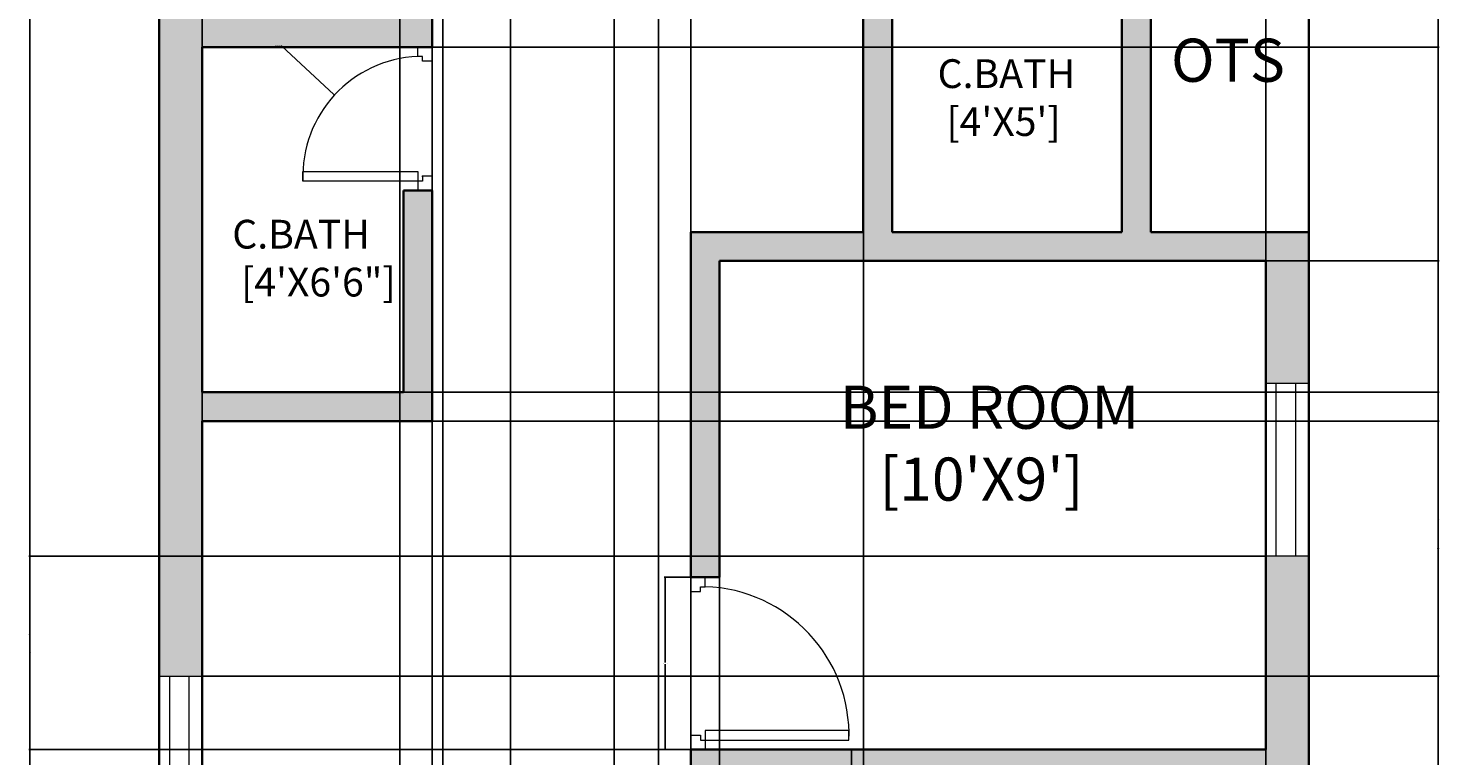
# Model space of a CAD drawing. Units: inches. Extents: x 1963 to 2258, y 1522 to 2116.
# Tile 2 of 3: x 1963 to 2257, y 1793 to 1945. Entities that reach past the tile are written whole.
import ezdxf

# ---------------------------------------------------------------- set-up
doc = ezdxf.new("R2010")
doc.units = ezdxf.units.IN
for name, color, linetype, lineweight in [('A-ANNO-DIMS', 2, 'Continuous', 18), ('A-AREA-IDEN', 7, 'Continuous', 18), ('A-DOOR', 3, 'Continuous', 18), ('A-GLAZ', 4, 'Continuous', 18), ('A-WALL', 7, 'Continuous', 35), ('A-WALL-PATT', 250, 'Continuous', 13)]:
    doc.layers.add(name, color=color, linetype=linetype, lineweight=lineweight)
doc.styles.get("Standard").update_dxf_attribs({"font": 'arial.ttf'})
doc.dimstyles.get("Standard").update_dxf_attribs({"dimtxt": 0.18, "dimasz": 0.18, "dimexe": 0.18, "dimexo": 0.0625, "dimgap": 0.09, "dimtad": 0, "dimtih": 1, "dimtoh": 1, "dimdec": 4, "dimzin": 0, "dimdsep": 46, "dimtxsty": 'Standard', "dimcen": 0.09, "dimadec": 0, "dimazin": 0, "dimtfac": 1, "dimtdec": 4, "dimtofl": 0, "dimtmove": 0, "dimatfit": 3, "dimfxl": 1, "dimtolj": 1, "dimtzin": 0, "dimarcsym": 0})

# ---------------------------------------------------------------- blocks, each defined once
blk = doc.blocks.new('WIN-36-9IN-WALL')
for p, q in [((-9, 0), (-9, 36.12)), ((-9, 36.12), (0, 36.12)), ((-6.81, 0), (-6.81, 36.12)), ((-4.5, 36.12), (-2.78, 36.12)), ((-2.78, 36.12), (-2.78, 0)), ((0, 36.12), (0, 0)), ((0, 0), (-9, 0)), ((-2.78, 0), (-6.81, 0)), ((0, 0), (-4.5, 0))]:
    blk.add_line(p, q)
blk = doc.blocks.new('DOOR-SWING-30IN')
for p, q in [((-3, -2), (-3, 0)), ((-3, 0), (0, 0)), ((-2, -2), (-3, -2)), ((-2, -3), (-2, -2)), ((0, 0), (0, -3)), ((0, 0), (0, -3)), ((0, -3), (-2, -3)), ((-27, -28), (-27, -26)), ((-27, -26), (-3, -26)), ((-3, -26), (-3, -28)), ((-3, -28), (-27, -28)), ((-2, -28), (-3, -28)), ((-3, -28), (-3, -30)), ((0, -27), (-2, -27)), ((-2, -27), (-2, -28)), ((0, -27), (0, -30)), ((-3, -30), (0, -30))]:
    blk.add_line(p, q)
blk.add_arc((-2, -27), 25.02, 92.2906, 182.2906)
blk = doc.blocks.new('DOOR-SWING-36IN')
for p, q in [((34, 33), (32, 33)), ((32, 33), (32, 3)), ((34, 3), (34, 33)), ((2, 3), (0, 3)), ((0, 3), (0, 0)), ((2, 2), (2, 3)), ((32, 3), (34, 3)), ((34, 2), (34, 3)), ((34, 3), (36, 3)), ((36, 3), (36, 0)), ((0, 0), (3, 0)), ((0, 0), (3, 0)), ((0, 0), (3, 0)), ((3, 2), (2, 2)), ((3, 0), (3, 2)), ((33, 0), (33, 2)), ((33, 2), (34, 2)), ((33, 0), (36, 0))]:
    blk.add_line(p, q)
blk.add_arc((33, 2), 31.02, 88.1524, 178.1524)
blk = doc.blocks.new('*D12')
at = {"layer": 'A-ANNO-DIMS', "color": 0, "lineweight": -2, "transparency": 16777216}
for p, q in [((2101.05, 1830.75), (2095.53, 1830.75)), ((2095.71, 1830.57), (2095.71, 1812.93)), ((2095.71, 1794.93), (2095.71, 1812.56)), ((2101.05, 1794.75), (2095.53, 1794.75))]:
    blk.add_line(p, q, dxfattribs=at)
at = {"layer": 'A-ANNO-DIMS', "color": 0, "transparency": 16777216}
for points in [[(2095.68, 1830.57), (2095.74, 1830.57), (2095.71, 1830.75)], [(2095.68, 1794.93), (2095.74, 1794.93), (2095.71, 1794.75)]]:
    blk.add_solid(points, dxfattribs=at)
at = {"layer": 'Defpoints', "color": 0, "transparency": 16777216}
for p in [(2101.11, 1830.75), (2095.71, 1794.75), (2101.11, 1794.75)]:
    blk.add_point(p, dxfattribs=at)
at = {"layer": 'A-ANNO-DIMS', "color": 0, "transparency": 16777216, "insert": (2095.71, 1812.75), "char_height": 0.18, "attachment_point": 5}
blk.add_mtext('\\A1;DOOR 36 TYP.', dxfattribs=at)
blk = doc.blocks.new('*D13')
at = {"layer": 'A-ANNO-DIMS', "color": 0, "lineweight": -2, "transparency": 16777216}
for p, q in [((2101.11, 1794.68), (2101.11, 1789.17)), ((2134.66, 1794.68), (2134.66, 1789.17)), ((2101.29, 1789.35), (2117.36, 1789.35)), ((2134.48, 1789.35), (2118.41, 1789.35))]:
    blk.add_line(p, q, dxfattribs=at)
at = {"layer": 'A-ANNO-DIMS', "color": 0, "transparency": 16777216}
for points in [[(2101.29, 1789.38), (2101.29, 1789.32), (2101.11, 1789.35)], [(2134.48, 1789.38), (2134.48, 1789.32), (2134.66, 1789.35)]]:
    blk.add_solid(points, dxfattribs=at)
at = {"layer": 'Defpoints', "color": 0, "transparency": 16777216}
for p in [(2101.11, 1794.75), (2134.66, 1794.75), (2134.66, 1789.35)]:
    blk.add_point(p, dxfattribs=at)
at = {"layer": 'A-ANNO-DIMS', "color": 0, "transparency": 16777216, "insert": (2117.89, 1789.35), "char_height": 0.18, "attachment_point": 5}
blk.add_mtext('\\A1;34 TYP.', dxfattribs=at)
blk = doc.blocks.new('*D15')
at = {"layer": 'A-ANNO-DIMS', "color": 0, "lineweight": -2, "transparency": 16777216}
for p, q in [((2094.32, 1548.81), (2094.32, 2115.96)), ((2221.11, 1548.81), (2221.11, 2115.96)), ((2094.5, 2115.78), (2157.26, 2115.78)), ((2220.93, 2115.78), (2158.17, 2115.78))]:
    blk.add_line(p, q, dxfattribs=at)
at = {"layer": 'A-ANNO-DIMS', "color": 0, "transparency": 16777216}
for points in [[(2094.5, 2115.81), (2094.5, 2115.75), (2094.32, 2115.78)], [(2220.93, 2115.81), (2220.93, 2115.75), (2221.11, 2115.78)]]:
    blk.add_solid(points, dxfattribs=at)
at = {"layer": 'Defpoints', "color": 0, "transparency": 16777216}
for p in [(2221.11, 2115.78), (2094.32, 1548.75), (2221.11, 1548.75)]:
    blk.add_point(p, dxfattribs=at)
at = {"layer": 'A-ANNO-DIMS', "color": 0, "transparency": 16777216, "insert": (2157.72, 2115.78), "char_height": 0.18, "attachment_point": 5}
blk.add_mtext('\\A1;126.79', dxfattribs=at)
blk = doc.blocks.new('*D18')
at = {"layer": 'A-ANNO-DIMS', "color": 0, "lineweight": -2, "transparency": 16777216}
for p, q in [((1999.11, 2079.68), (1999.11, 1521.53)), ((2101.11, 2079.68), (2101.11, 1521.53)), ((1999.29, 1521.71), (2049.83, 1521.71)), ((2100.93, 1521.71), (2050.39, 1521.71))]:
    blk.add_line(p, q, dxfattribs=at)
at = {"layer": 'A-ANNO-DIMS', "color": 0, "transparency": 16777216}
for points in [[(1999.29, 1521.74), (1999.29, 1521.68), (1999.11, 1521.71)], [(2100.93, 1521.74), (2100.93, 1521.68), (2101.11, 1521.71)]]:
    blk.add_solid(points, dxfattribs=at)
at = {"layer": 'Defpoints', "color": 0, "transparency": 16777216}
for p in [(1999.11, 2079.75), (2101.11, 2079.75), (2101.11, 1521.71)]:
    blk.add_point(p, dxfattribs=at)
at = {"layer": 'A-ANNO-DIMS', "color": 0, "transparency": 16777216, "insert": (2050.11, 1521.71), "char_height": 0.18, "attachment_point": 5}
blk.add_mtext('\\A1;102', dxfattribs=at)
blk = doc.blocks.new('*D23')
at = {"layer": 'A-ANNO-DIMS', "color": 0, "lineweight": -2, "transparency": 16777216}
for p, q in [((1999.17, 1863.32), (2257.32, 1863.32)), ((2257.14, 1863.14), (2257.14, 1836.88)), ((2257.14, 1810.25), (2257.14, 1836.52)), ((1999.17, 1810.07), (2257.32, 1810.07))]:
    blk.add_line(p, q, dxfattribs=at)
at = {"layer": 'A-ANNO-DIMS', "color": 0, "transparency": 16777216}
for points in [[(2257.11, 1863.14), (2257.17, 1863.14), (2257.14, 1863.32)], [(2257.11, 1810.25), (2257.17, 1810.25), (2257.14, 1810.07)]]:
    blk.add_solid(points, dxfattribs=at)
at = {"layer": 'Defpoints', "color": 0, "transparency": 16777216}
for p in [(1999.11, 1863.32), (2257.14, 1863.32), (1999.11, 1810.07)]:
    blk.add_point(p, dxfattribs=at)
at = {"layer": 'A-ANNO-DIMS', "color": 0, "transparency": 16777216, "insert": (2257.14, 1836.7), "char_height": 0.18, "attachment_point": 5}
blk.add_mtext('\\A1;53.25', dxfattribs=at)
blk = doc.blocks.new('*D24')
at = {"layer": 'A-ANNO-DIMS', "color": 0, "lineweight": -2, "transparency": 16777216}
for p, q in [((1999.17, 1941.32), (2257.32, 1941.32)), ((2257.14, 1941.14), (2257.14, 1905.5)), ((2257.14, 1869.5), (2257.14, 1905.14)), ((1999.17, 1869.32), (2257.32, 1869.32))]:
    blk.add_line(p, q, dxfattribs=at)
at = {"layer": 'A-ANNO-DIMS', "color": 0, "transparency": 16777216}
for points in [[(2257.11, 1941.14), (2257.17, 1941.14), (2257.14, 1941.32)], [(2257.11, 1869.5), (2257.17, 1869.5), (2257.14, 1869.32)]]:
    blk.add_solid(points, dxfattribs=at)
at = {"layer": 'Defpoints', "color": 0, "transparency": 16777216}
for p in [(1999.11, 1941.32), (2257.14, 1941.32), (1999.11, 1869.32)]:
    blk.add_point(p, dxfattribs=at)
at = {"layer": 'A-ANNO-DIMS', "color": 0, "transparency": 16777216, "insert": (2257.14, 1905.32), "char_height": 0.18, "attachment_point": 5}
blk.add_mtext('\\A1;72', dxfattribs=at)
blk = doc.blocks.new('*D28')
at = {"layer": 'A-ANNO-DIMS', "color": 0, "lineweight": -2, "transparency": 16777216}
for p, q in [((2221.17, 1896.75), (2257.32, 1896.75)), ((2257.14, 1896.57), (2257.14, 1842.93)), ((2257.14, 1788.93), (2257.14, 1842.57)), ((2221.17, 1788.75), (2257.32, 1788.75))]:
    blk.add_line(p, q, dxfattribs=at)
at = {"layer": 'A-ANNO-DIMS', "color": 0, "transparency": 16777216}
for points in [[(2257.11, 1896.57), (2257.17, 1896.57), (2257.14, 1896.75)], [(2257.11, 1788.93), (2257.17, 1788.93), (2257.14, 1788.75)]]:
    blk.add_solid(points, dxfattribs=at)
at = {"layer": 'Defpoints', "color": 0, "transparency": 16777216}
for p in [(2221.11, 1896.75), (2257.14, 1896.75), (2221.11, 1788.75)]:
    blk.add_point(p, dxfattribs=at)
at = {"layer": 'A-ANNO-DIMS', "color": 0, "transparency": 16777216, "insert": (2257.14, 1842.75), "char_height": 0.18, "attachment_point": 5}
blk.add_mtext('\\A1;108', dxfattribs=at)
blk = doc.blocks.new('*D29')
at = {"layer": 'A-ANNO-DIMS', "color": 0, "lineweight": -2, "transparency": 16777216}
for p, q in [((2230.17, 1971.75), (2257.32, 1971.75)), ((2257.14, 1971.57), (2257.14, 1934.43)), ((2257.14, 1896.93), (2257.14, 1934.07)), ((2221.17, 1896.75), (2257.32, 1896.75))]:
    blk.add_line(p, q, dxfattribs=at)
at = {"layer": 'A-ANNO-DIMS', "color": 0, "transparency": 16777216}
for points in [[(2257.11, 1971.57), (2257.17, 1971.57), (2257.14, 1971.75)], [(2257.11, 1896.93), (2257.17, 1896.93), (2257.14, 1896.75)]]:
    blk.add_solid(points, dxfattribs=at)
at = {"layer": 'Defpoints', "color": 0, "transparency": 16777216}
for p in [(2230.11, 1971.75), (2257.14, 1971.75), (2221.11, 1896.75)]:
    blk.add_point(p, dxfattribs=at)
at = {"layer": 'A-ANNO-DIMS', "color": 0, "transparency": 16777216, "insert": (2257.14, 1934.25), "char_height": 0.18, "attachment_point": 5}
blk.add_mtext('\\A1;75', dxfattribs=at)
blk = doc.blocks.new('*D31')
at = {"layer": 'A-ANNO-DIMS', "color": 0, "lineweight": -2, "transparency": 16777216}
for p, q in [((2221.05, 1835.13), (1962.89, 1835.13)), ((1963.07, 1834.95), (1963.07, 1815.12)), ((1963.07, 1794.93), (1963.07, 1814.75)), ((2221.05, 1794.75), (1962.89, 1794.75))]:
    blk.add_line(p, q, dxfattribs=at)
at = {"layer": 'A-ANNO-DIMS', "color": 0, "transparency": 16777216}
for points in [[(1963.04, 1834.95), (1963.1, 1834.95), (1963.07, 1835.13)], [(1963.04, 1794.93), (1963.1, 1794.93), (1963.07, 1794.75)]]:
    blk.add_solid(points, dxfattribs=at)
at = {"layer": 'Defpoints', "color": 0, "transparency": 16777216}
for p in [(2221.11, 1835.13), (1963.07, 1794.75), (2221.11, 1794.75)]:
    blk.add_point(p, dxfattribs=at)
at = {"layer": 'A-ANNO-DIMS', "color": 0, "transparency": 16777216, "insert": (1963.07, 1814.94), "char_height": 0.18, "attachment_point": 5}
blk.add_mtext('\\A1;40.38', dxfattribs=at)
blk = doc.blocks.new('*D33')
at = {"layer": 'A-ANNO-DIMS', "color": 0, "lineweight": -2, "transparency": 16777216}
for p, q in [((1999.11, 1863.26), (1999.11, 1521.53)), ((2047.11, 1863.26), (2047.11, 1521.53)), ((1999.29, 1521.71), (2022.89, 1521.71)), ((2046.93, 1521.71), (2023.33, 1521.71))]:
    blk.add_line(p, q, dxfattribs=at)
at = {"layer": 'A-ANNO-DIMS', "color": 0, "transparency": 16777216}
for points in [[(1999.29, 1521.74), (1999.29, 1521.68), (1999.11, 1521.71)], [(2046.93, 1521.74), (2046.93, 1521.68), (2047.11, 1521.71)]]:
    blk.add_solid(points, dxfattribs=at)
at = {"layer": 'Defpoints', "color": 0, "transparency": 16777216}
for p in [(1999.11, 1863.32), (2047.11, 1863.32), (2047.11, 1521.71)]:
    blk.add_point(p, dxfattribs=at)
at = {"layer": 'A-ANNO-DIMS', "color": 0, "transparency": 16777216, "insert": (2023.11, 1521.71), "char_height": 0.18, "attachment_point": 5}
blk.add_mtext('\\A1;48', dxfattribs=at)
blk = doc.blocks.new('*D34')
at = {"layer": 'A-ANNO-DIMS', "color": 0, "lineweight": -2, "transparency": 16777216}
for p, q in [((2047.11, 1971.68), (2047.11, 1521.53)), ((2137.11, 1971.68), (2137.11, 1521.53)), ((2047.29, 1521.71), (2091.89, 1521.71)), ((2136.93, 1521.71), (2092.33, 1521.71))]:
    blk.add_line(p, q, dxfattribs=at)
at = {"layer": 'A-ANNO-DIMS', "color": 0, "transparency": 16777216}
for points in [[(2047.29, 1521.74), (2047.29, 1521.68), (2047.11, 1521.71)], [(2136.93, 1521.74), (2136.93, 1521.68), (2137.11, 1521.71)]]:
    blk.add_solid(points, dxfattribs=at)
at = {"layer": 'Defpoints', "color": 0, "transparency": 16777216}
for p in [(2047.11, 1971.75), (2137.11, 1971.75), (2137.11, 1521.71)]:
    blk.add_point(p, dxfattribs=at)
at = {"layer": 'A-ANNO-DIMS', "color": 0, "transparency": 16777216, "insert": (2092.11, 1521.71), "char_height": 0.18, "attachment_point": 5}
blk.add_mtext('\\A1;90', dxfattribs=at)
blk = doc.blocks.new('*D35')
at = {"layer": 'A-ANNO-DIMS', "color": 0, "lineweight": -2, "transparency": 16777216}
for p, q in [((2197.11, 1902.81), (2197.11, 2115.96)), ((2230.11, 1902.81), (2230.11, 2115.96)), ((2197.29, 2115.78), (2213.39, 2115.78)), ((2229.93, 2115.78), (2213.83, 2115.78))]:
    blk.add_line(p, q, dxfattribs=at)
at = {"layer": 'A-ANNO-DIMS', "color": 0, "transparency": 16777216}
for points in [[(2197.29, 2115.81), (2197.29, 2115.75), (2197.11, 2115.78)], [(2229.93, 2115.81), (2229.93, 2115.75), (2230.11, 2115.78)]]:
    blk.add_solid(points, dxfattribs=at)
at = {"layer": 'Defpoints', "color": 0, "transparency": 16777216}
for p in [(2230.11, 2115.78), (2197.11, 1902.75), (2230.11, 1902.75)]:
    blk.add_point(p, dxfattribs=at)
at = {"layer": 'A-ANNO-DIMS', "color": 0, "transparency": 16777216, "insert": (2213.61, 2115.78), "char_height": 0.18, "attachment_point": 5}
blk.add_mtext('\\A1;33', dxfattribs=at)
blk = doc.blocks.new('*D36')
at = {"layer": 'A-ANNO-DIMS', "color": 0, "lineweight": -2, "transparency": 16777216}
for p, q in [((2143.11, 1902.81), (2143.11, 2115.96)), ((2191.11, 1902.81), (2191.11, 2115.96)), ((2143.29, 2115.78), (2166.89, 2115.78)), ((2190.93, 2115.78), (2167.33, 2115.78))]:
    blk.add_line(p, q, dxfattribs=at)
at = {"layer": 'A-ANNO-DIMS', "color": 0, "transparency": 16777216}
for points in [[(2143.29, 2115.81), (2143.29, 2115.75), (2143.11, 2115.78)], [(2190.93, 2115.81), (2190.93, 2115.75), (2191.11, 2115.78)]]:
    blk.add_solid(points, dxfattribs=at)
at = {"layer": 'Defpoints', "color": 0, "transparency": 16777216}
for p in [(2143.11, 2115.78), (2143.11, 1902.75), (2191.11, 1902.75)]:
    blk.add_point(p, dxfattribs=at)
at = {"layer": 'A-ANNO-DIMS', "color": 0, "transparency": 16777216, "insert": (2167.11, 2115.78), "char_height": 0.18, "attachment_point": 5}
blk.add_mtext('\\A1;48', dxfattribs=at)
blk = doc.blocks.new('*D37')
at = {"layer": 'A-ANNO-DIMS', "color": 0, "lineweight": -2, "transparency": 16777216}
for p, q in [((1999.11, 1743.38), (1999.11, 2115.96)), ((2063.45, 1743.38), (2063.45, 2115.96)), ((1999.29, 2115.78), (2030.89, 2115.78)), ((2063.27, 2115.78), (2031.67, 2115.78))]:
    blk.add_line(p, q, dxfattribs=at)
at = {"layer": 'A-ANNO-DIMS', "color": 0, "transparency": 16777216}
for points in [[(1999.29, 2115.81), (1999.29, 2115.75), (1999.11, 2115.78)], [(2063.27, 2115.81), (2063.27, 2115.75), (2063.45, 2115.78)]]:
    blk.add_solid(points, dxfattribs=at)
at = {"layer": 'Defpoints', "color": 0, "transparency": 16777216}
for p in [(2063.45, 2115.78), (1999.11, 1743.32), (2063.45, 1743.32)]:
    blk.add_point(p, dxfattribs=at)
at = {"layer": 'A-ANNO-DIMS', "color": 0, "transparency": 16777216, "insert": (2031.28, 2115.78), "char_height": 0.18, "attachment_point": 5}
blk.add_mtext('\\A1;64.34', dxfattribs=at)
blk = doc.blocks.new('*D38')
at = {"layer": 'A-ANNO-DIMS', "color": 0, "lineweight": -2, "transparency": 16777216}
for p, q in [((1999.11, 1647.38), (1999.11, 2115.96)), ((2049.32, 1647.35), (2049.32, 2115.96)), ((1999.29, 2115.78), (2023.84, 2115.78)), ((2049.14, 2115.78), (2024.59, 2115.78))]:
    blk.add_line(p, q, dxfattribs=at)
at = {"layer": 'A-ANNO-DIMS', "color": 0, "transparency": 16777216}
for points in [[(1999.29, 2115.81), (1999.29, 2115.75), (1999.11, 2115.78)], [(2049.14, 2115.81), (2049.14, 2115.75), (2049.32, 2115.78)]]:
    blk.add_solid(points, dxfattribs=at)
at = {"layer": 'Defpoints', "color": 0, "transparency": 16777216}
for p in [(2049.32, 2115.78), (1999.11, 1647.32), (2049.32, 1647.29)]:
    blk.add_point(p, dxfattribs=at)
at = {"layer": 'A-ANNO-DIMS', "color": 0, "transparency": 16777216, "insert": (2024.22, 2115.78), "char_height": 0.18, "attachment_point": 5}
blk.add_mtext('\\A1;50.21', dxfattribs=at)
blk = doc.blocks.new('*D42')
at = {"layer": 'A-ANNO-DIMS', "color": 0, "lineweight": -2, "transparency": 16777216}
for p, q in [((1999.11, 1557.81), (1999.11, 2115.96)), ((2040.32, 1557.81), (2040.32, 2115.96)), ((1999.29, 2115.78), (2019.25, 2115.78)), ((2040.14, 2115.78), (2020.18, 2115.78))]:
    blk.add_line(p, q, dxfattribs=at)
at = {"layer": 'A-ANNO-DIMS', "color": 0, "transparency": 16777216}
for points in [[(1999.29, 2115.81), (1999.29, 2115.75), (1999.11, 2115.78)], [(2040.14, 2115.81), (2040.14, 2115.75), (2040.32, 2115.78)]]:
    blk.add_solid(points, dxfattribs=at)
at = {"layer": 'Defpoints', "color": 0, "transparency": 16777216}
for p in [(2040.32, 2115.78), (1999.11, 1557.75), (2040.32, 1557.75)]:
    blk.add_point(p, dxfattribs=at)
at = {"layer": 'A-ANNO-DIMS', "color": 0, "transparency": 16777216, "insert": (2019.72, 2115.78), "char_height": 0.18, "attachment_point": 5}
blk.add_mtext('\\A1;41.214', dxfattribs=at)
blk = doc.blocks.new('*D43')
at = {"layer": 'A-ANNO-DIMS', "color": 0, "lineweight": -2, "transparency": 16777216}
for p, q in [((2040.32, 1557.81), (2040.32, 2115.96)), ((2049.32, 1557.81), (2049.32, 2115.96)), ((2040.5, 2115.78), (2044.67, 2115.78)), ((2049.14, 2115.78), (2044.97, 2115.78))]:
    blk.add_line(p, q, dxfattribs=at)
at = {"layer": 'A-ANNO-DIMS', "color": 0, "transparency": 16777216}
for points in [[(2040.5, 2115.81), (2040.5, 2115.75), (2040.32, 2115.78)], [(2049.14, 2115.81), (2049.14, 2115.75), (2049.32, 2115.78)]]:
    blk.add_solid(points, dxfattribs=at)
at = {"layer": 'Defpoints', "color": 0, "transparency": 16777216}
for p in [(2049.32, 2115.78), (2040.32, 1557.75), (2049.32, 1557.75)]:
    blk.add_point(p, dxfattribs=at)
at = {"layer": 'A-ANNO-DIMS', "color": 0, "transparency": 16777216, "insert": (2044.82, 2115.78), "char_height": 0.18, "attachment_point": 5}
blk.add_mtext('\\A1;9', dxfattribs=at)
blk = doc.blocks.new('*D45')
at = {"layer": 'A-ANNO-DIMS', "color": 0, "lineweight": -2, "transparency": 16777216}
for p, q in [((2107.11, 1896.68), (2107.11, 1521.53)), ((2221.11, 1896.68), (2221.11, 1521.53)), ((2107.29, 1521.71), (2163.83, 1521.71)), ((2220.93, 1521.71), (2164.39, 1521.71))]:
    blk.add_line(p, q, dxfattribs=at)
at = {"layer": 'A-ANNO-DIMS', "color": 0, "transparency": 16777216}
for points in [[(2107.29, 1521.74), (2107.29, 1521.68), (2107.11, 1521.71)], [(2220.93, 1521.74), (2220.93, 1521.68), (2221.11, 1521.71)]]:
    blk.add_solid(points, dxfattribs=at)
at = {"layer": 'Defpoints', "color": 0, "transparency": 16777216}
for p in [(2107.11, 1896.75), (2221.11, 1896.75), (2221.11, 1521.71)]:
    blk.add_point(p, dxfattribs=at)
at = {"layer": 'A-ANNO-DIMS', "color": 0, "transparency": 16777216, "insert": (2164.11, 1521.71), "char_height": 0.18, "attachment_point": 5}
blk.add_mtext('\\A1;114', dxfattribs=at)
blk = doc.blocks.new('*D46')
at = {"layer": 'A-ANNO-DIMS', "color": 0, "lineweight": -2, "transparency": 16777216}
for p, q in [((2085.06, 1647.35), (2085.06, 2115.96)), ((2101.11, 1647.38), (2101.11, 2115.96)), ((2085.24, 2115.78), (2092.7, 2115.78)), ((2100.93, 2115.78), (2093.47, 2115.78))]:
    blk.add_line(p, q, dxfattribs=at)
at = {"layer": 'A-ANNO-DIMS', "color": 0, "transparency": 16777216}
for points in [[(2085.24, 2115.81), (2085.24, 2115.75), (2085.06, 2115.78)], [(2100.93, 2115.81), (2100.93, 2115.75), (2101.11, 2115.78)]]:
    blk.add_solid(points, dxfattribs=at)
at = {"layer": 'Defpoints', "color": 0, "transparency": 16777216}
for p in [(2101.11, 2115.78), (2085.06, 1647.29), (2101.11, 1647.32)]:
    blk.add_point(p, dxfattribs=at)
at = {"layer": 'A-ANNO-DIMS', "color": 0, "transparency": 16777216, "insert": (2093.08, 2115.78), "char_height": 0.18, "attachment_point": 5}
blk.add_mtext('\\A1;16.05', dxfattribs=at)
blk = doc.blocks.new('*D47')
at = {"layer": 'A-ANNO-DIMS', "color": 0, "lineweight": -2, "transparency": 16777216}
for p, q in [((1990.05, 2088.75), (1962.89, 2088.75)), ((1963.07, 2088.57), (1963.07, 1818.93)), ((1963.07, 1548.93), (1963.07, 1818.57)), ((1990.05, 1548.75), (1962.89, 1548.75))]:
    blk.add_line(p, q, dxfattribs=at)
at = {"layer": 'A-ANNO-DIMS', "color": 0, "transparency": 16777216}
for points in [[(1963.04, 2088.57), (1963.1, 2088.57), (1963.07, 2088.75)], [(1963.04, 1548.93), (1963.1, 1548.93), (1963.07, 1548.75)]]:
    blk.add_solid(points, dxfattribs=at)
at = {"layer": 'Defpoints', "color": 0, "transparency": 16777216}
for p in [(1963.07, 2088.75), (1990.11, 2088.75), (1990.11, 1548.75)]:
    blk.add_point(p, dxfattribs=at)
at = {"layer": 'A-ANNO-DIMS', "color": 0, "transparency": 16777216, "insert": (1963.07, 1818.75), "char_height": 0.18, "attachment_point": 5}
blk.add_mtext('\\A1;540', dxfattribs=at)
blk = doc.blocks.new('*D49')
at = {"layer": 'A-ANNO-DIMS', "color": 0, "lineweight": -2, "transparency": 16777216}
for p, q in [((2015.51, 1941.56), (2015.69, 1941.56)), ((2015.69, 1941.56), (2026.59, 1931.5)), ((2045.02, 1914.41), (2045.2, 1914.41)), ((2045.11, 1914.32), (2045.11, 1914.5))]:
    blk.add_line(p, q, dxfattribs=at)
at = {"layer": 'A-ANNO-DIMS', "color": 0, "transparency": 16777216}
blk.add_solid([(2026.61, 1931.53), (2026.57, 1931.48), (2026.72, 1931.38)], dxfattribs=at)
at = {"layer": 'Defpoints', "color": 0, "transparency": 16777216}
for p in [(2026.72, 1931.38), (2045.11, 1914.41)]:
    blk.add_point(p, dxfattribs=at)
at = {"layer": 'A-ANNO-DIMS', "color": 0, "transparency": 16777216, "insert": (2014.84, 1941.56), "char_height": 0.18, "attachment_point": 5}
blk.add_mtext('\\A1;2X R25.02', dxfattribs=at)

msp = doc.modelspace()

# ---------------------------------------------------------------- hatches: boundary and pattern name
at = {"layer": 'A-WALL-PATT'}
h = msp.add_hatch(color=256, dxfattribs=at)
h.dxf.hatch_style = 1
h.paths.add_polyline_path([(2040.4282, 2088.7475), (1990.109, 2088.7475), (1990.109, 2047.2372), (1999.109, 2047.2372), (1999.109, 2079.7475), (2040.4282, 2079.7475)])
h.paths.add_polyline_path([(2159.691, 2088.7475), (2076.5488, 2088.7475), (2076.5488, 2084.2475), (2076.5488, 2079.7475), (2101.109, 2079.7475), (2101.109, 1977.7475), (2101.109, 1971.7475), (2107.109, 1971.7475), (2107.109, 1974.7475), (2107.109, 1977.7475), (2107.109, 2079.7475), (2110.109, 2079.7475), (2159.691, 2079.7475)])
h.paths.add_polyline_path([(2230.109, 2088.7475), (2195.8116, 2088.7475), (2195.8116, 2084.2475), (2195.8116, 2079.7475), (2221.109, 2079.7475), (2221.109, 2045.7556), (2230.109, 2045.7556)])
h.paths.add_polyline_path([(2230.109, 2009.6349), (2225.609, 2009.6349), (2221.109, 2009.6349), (2221.109, 1977.7475), (2173.109, 1977.7475), (2173.109, 1974.7475), (2173.0802, 1971.7475), (2178.9852, 1971.7475), (2185.109, 1971.7475), (2191.109, 1971.7475), (2191.109, 1902.7475), (2143.109, 1902.7475), (2143.109, 1971.7475), (2143.109, 1977.7475), (2137.109, 1977.7475), (2137.109, 1971.7475), (2137.109, 1902.7475), (2101.109, 1902.7475), (2101.109, 1830.7475), (2104.109, 1830.7475), (2107.109, 1830.7475), (2107.109, 1896.7475), (2221.109, 1896.7475), (2221.109, 1871.2465), (2230.109, 1871.2465), (2230.109, 1902.7475), (2197.109, 1902.7475), (2197.109, 1971.7475), (2230.109, 1971.7475)])
h.paths.add_polyline_path([(2065.109, 1977.7475), (1999.109, 1977.7475), (1999.109, 2011.1166), (1994.609, 2011.1166), (1990.109, 2011.1166), (1990.109, 1810.0744), (1999.109, 1810.0744), (1999.109, 1863.32), (2047.109, 1863.32), (2047.109, 1869.32), (2047.109, 1911.4119), (2044.109, 1911.4119), (2041.109, 1911.4119), (2041.109, 1869.32), (1999.109, 1869.32), (1999.109, 1941.32), (2041.109, 1941.32), (2044.109, 1941.32), (2044.109, 1941.4119), (2047.109, 1941.4119), (2047.109, 1971.7475), (2065.109, 1971.7475), (2065.109, 1974.7475)])
h.paths.add_polyline_path([(2041.109, 1971.7475), (2041.109, 1947.32), (1999.109, 1947.32), (1999.109, 1971.7475)], flags=16)
h.paths.add_polyline_path([(2230.109, 1835.1259), (2225.609, 1835.1259), (2221.109, 1835.1259), (2221.109, 1794.7475), (2101.109, 1794.7475), (2101.109, 1788.7475), (2221.109, 1788.7475), (2221.109, 1763.2023), (2230.109, 1763.2023)])
h.paths.add_polyline_path([(2063.4524, 1743.32), (1999.109, 1743.32), (1999.109, 1773.9538), (1994.609, 1773.9538), (1992.3007, 1773.9538), (1990.109, 1773.9538), (1990.109, 1703.9859), (1999.109, 1703.9859), (1999.109, 1737.32), (2063.4524, 1737.32)])
h.paths.add_polyline_path([(2169.7564, 1696.9689), (2169.7564, 1698.7475), (2143.109, 1698.7475), (2143.109, 1692.7475), (2143.6022, 1692.7475), (2169.7564, 1692.7475), (2169.7564, 1695.7336)])
h.paths.add_polyline_path([(2230.109, 1727.0817), (2225.609, 1727.0817), (2221.109, 1727.0817), (2221.109, 1698.7475), (2205.4934, 1698.7475), (2205.4934, 1692.7475), (2221.109, 1692.7475), (2221.109, 1557.7475), (2221.109, 1548.7475), (2230.109, 1548.7475)])
h.paths.add_polyline_path([(2107.109, 1760.0903), (2101.109, 1760.0903), (2101.109, 1743.32), (2101.109, 1737.32), (2101.109, 1698.7475), (2101.109, 1687.7398), (2104.1229, 1687.7398), (2105.3583, 1687.7398), (2107.109, 1687.7398), (2107.109, 1692.7475), (2107.109, 1695.7475), (2107.109, 1698.7475)])
h.paths.add_polyline_path([(2107.109, 1652.0028), (2101.109, 1652.0028), (2101.109, 1647.32), (2085.0601, 1647.32), (2085.0601, 1641.32), (2085.3232, 1641.32), (2107.109, 1641.32)])
h.paths.add_polyline_path([(2049.3232, 1645.5414), (2049.3232, 1647.32), (1999.109, 1647.32), (1999.109, 1667.8653), (1994.609, 1667.8653), (1992.3007, 1667.8653), (1990.109, 1667.8653), (1990.109, 1548.7475), (2094.3232, 1548.7475), (2094.3232, 1557.7475), (2085.3232, 1557.7475), (1999.109, 1557.7475), (1999.109, 1641.32), (2049.3232, 1641.32), (2049.3232, 1644.306)])

# ---------------------------------------------------------------- linework, layer by layer
at = {"layer": 'A-WALL'}
for p, q in [((2047.109, 1941.32), (2047.109, 1971.7475)), ((2137.109, 1902.7475), (2137.109, 1971.7475)), ((2143.109, 1902.7475), (2143.109, 1971.7475)), ((2191.109, 1902.7475), (2191.109, 1971.7475)), ((2197.109, 1902.7475), (2197.109, 1971.7475)), ((2041.109, 1941.32), (1999.109, 1941.32)), ((2041.109, 1941.32), (2047.109, 1941.32)), ((2041.109, 1869.32), (2041.109, 1911.4119)), ((2047.109, 1911.4119), (2041.109, 1911.4119)), ((2047.109, 1869.32), (2047.109, 1911.4119)), ((2101.109, 1902.7475), (2101.109, 1869.32)), ((2101.109, 1902.7475), (2101.109, 1830.7475)), ((2137.109, 1902.7475), (2101.109, 1902.7475)), ((2161.109, 1902.7475), (2143.109, 1902.7475)), ((2178.9852, 1902.7475), (2143.109, 1902.7475)), ((2143.109, 1902.7475), (2191.109, 1902.7475)), ((2178.9852, 1902.7475), (2161.109, 1902.7475)), ((2191.109, 1902.7475), (2184.9852, 1902.7475)), ((2230.109, 1902.7475), (2197.109, 1902.7475)), ((2221.109, 1896.7475), (2107.109, 1896.7475)), ((2107.109, 1830.7475), (2107.109, 1896.7475)), ((2221.109, 1794.7475), (2221.109, 1896.7475)), ((1999.109, 1869.32), (2041.109, 1869.32)), ((1999.109, 1869.32), (2041.109, 1869.32)), ((2047.109, 1869.32), (2047.109, 1863.32)), ((1999.109, 1743.32), (1999.109, 1863.32)), ((1999.109, 1863.32), (2047.109, 1863.32)), ((2101.109, 1830.7475), (2107.109, 1830.7475)), ((2221.109, 1794.7475), (2101.109, 1794.7475)), ((2221.109, 1794.7475), (2107.109, 1794.7475))]:
    msp.add_line(p, q, dxfattribs=at)
for points in [[(1990.109, 2088.7475), (2230.109, 2088.7475), (2230.109, 1548.7475), (1990.109, 1548.7475), (1990.109, 2088.7475)], [(1999.109, 1869.32), (1999.109, 1941.32)], [(2221.109, 1896.7475), (2221.109, 1794.7475)], [(1999.109, 1743.32), (1999.109, 1863.32)], [(2221.109, 1794.7475), (2101.109, 1794.7475), (2101.109, 1788.7475), (2221.109, 1788.7475)]]:
    msp.add_lwpolyline(points, dxfattribs=at)

# ---------------------------------------------------------------- block references
at = {"layer": 'A-DOOR'}
msp.add_blockref('DOOR-SWING-30IN', (2047.109, 1941.4119), dxfattribs=at)
at = {"layer": 'A-DOOR', "rotation": 269.9999999999987}
msp.add_blockref('DOOR-SWING-36IN', (2101.109, 1830.7475), dxfattribs=at)
at = {"layer": 'A-GLAZ'}
for p in [(2230.109, 1835.1259), (1999.109, 1773.9538)]:
    msp.add_blockref('WIN-36-9IN-WALL', p, dxfattribs=at)

# ---------------------------------------------------------------- texts
at = {"layer": 'A-AREA-IDEN', "attachment_point": 1}
for s, width, heights, insert, char_height in [('OTS', 32.745855, [0], (2201.3472, 1943.1278), 9), ("C.BATH\\P [4'X5']", 38.951704, [25.9925], (2152.6072, 1938.8282), 6), ('C.BATH\\P [4\'X6\'6"]', 38.951704, [25.9925], (2005.3607, 1905.32), 6), ("BED ROOM\\P   [10'X9']", 73.304435, [38.0827], (2132.2117, 1870.7008), 9)]:
    msp.add_mtext_dynamic_manual_height_columns(s, width=width, gutter_width=12.5, heights=heights, dxfattribs=dict(at, insert=insert, char_height=char_height))

# ---------------------------------------------------------------- dimensions: what is measured, and where the dimension line sits
at = {"layer": 'A-ANNO-DIMS'}
for base, p1, p2, override, picture, middle in [((2063.4524, 2115.7825), (1999.109, 1743.32), (2063.4524, 1743.32), {"dimdec": 2, "dimlfac": 1, "dimrnd": 0, "dimzin": 0, "dimdsep": 46, "dimlunit": 2}, '*D37', (2031.2807, 2115.7825)), ((2049.3232, 2115.7825), (1999.109, 1647.32), (2049.3232, 1647.2921), {"dimdec": 2, "dimlfac": 1, "dimrnd": 0, "dimzin": 0, "dimdsep": 46, "dimlunit": 2}, '*D38', (2024.2161, 2115.7825)), ((2040.3232, 2115.7825), (1999.109, 1557.7475), (2040.3232, 1557.7475), {"dimdec": 3, "dimlfac": 1, "dimrnd": 0, "dimzin": 0, "dimdsep": 46, "dimlunit": 2}, '*D42', (2019.7161, 2115.7825)), ((2049.3232, 2115.7825), (2040.3232, 1557.7475), (2049.3232, 1557.7475), {"dimdec": 0, "dimlfac": 1, "dimrnd": 0, "dimzin": 0, "dimdsep": 46, "dimlunit": 2}, '*D43', (2044.8232, 2115.7825)), ((2101.109, 2115.7825), (2085.0601, 1647.2921), (2101.109, 1647.32), {"dimdec": 2, "dimlfac": 1, "dimrnd": 0, "dimzin": 0, "dimdsep": 46, "dimlunit": 2}, '*D46', (2093.0846, 2115.7825)), ((2221.109, 2115.7825), (2094.3232, 1548.7475), (2221.109, 1548.7475), {"dimdec": 2, "dimlfac": 1, "dimrnd": 0, "dimzin": 0, "dimdsep": 46, "dimlunit": 2}, '*D15', (2157.7161, 2115.7825)), ((2143.109, 2115.7825), (2191.109, 1902.7475), (2143.109, 1902.7475), {"dimdec": 0, "dimlfac": 1, "dimrnd": 0, "dimzin": 0, "dimdsep": 46, "dimlunit": 2}, '*D36', (2167.109, 2115.7825)), ((2230.109, 2115.7825), (2197.109, 1902.7475), (2230.109, 1902.7475), {"dimdec": 0, "dimlfac": 1, "dimrnd": 0, "dimzin": 0, "dimdsep": 46, "dimlunit": 2}, '*D35', (2213.609, 2115.7825)), ((2101.109, 1521.7125), (1999.109, 2079.7475), (2101.109, 2079.7475), {"dimdec": 0, "dimlfac": 1, "dimrnd": 0, "dimzin": 0, "dimdsep": 46, "dimlunit": 2}, '*D18', (2050.109, 1521.7125)), ((2137.109, 1521.7125), (2047.109, 1971.7475), (2137.109, 1971.7475), {"dimdec": 0, "dimlfac": 1, "dimrnd": 0, "dimzin": 0, "dimdsep": 46, "dimlunit": 2}, '*D34', (2092.109, 1521.7125)), ((2221.109, 1521.7125), (2107.109, 1896.7475), (2221.109, 1896.7475), {"dimdec": 0, "dimlfac": 1, "dimrnd": 0, "dimzin": 0, "dimdsep": 46, "dimlunit": 2}, '*D45', (2164.109, 1521.7125)), ((2047.109, 1521.7125), (1999.109, 1863.32), (2047.109, 1863.32), {"dimdec": 0, "dimlfac": 1, "dimrnd": 0, "dimzin": 0, "dimdsep": 46, "dimlunit": 2}, '*D33', (2023.109, 1521.7125))]:
    dim = msp.add_linear_dim(base=base, p1=p1, p2=p2, dimstyle='Standard', override=override, dxfattribs=at)
    dim.commit()
    dim.dimension.update_dxf_attribs({"geometry": picture, "text_midpoint": middle})
for base, p1, p2, override, picture, middle in [((1963.074, 2088.7475), (1990.109, 1548.7475), (1990.109, 2088.7475), {"dimdec": 0, "dimlfac": 1, "dimrnd": 0, "dimzin": 0, "dimdsep": 46, "dimlunit": 2}, '*D47', (1963.074, 1818.7475)), ((2257.144, 1971.7475), (2221.109, 1896.7475), (2230.109, 1971.7475), {"dimdec": 0, "dimlfac": 1, "dimrnd": 0, "dimzin": 0, "dimdsep": 46, "dimlunit": 2}, '*D29', (2257.144, 1934.2475)), ((2257.144, 1941.32), (1999.109, 1869.32), (1999.109, 1941.32), {"dimdec": 0, "dimlfac": 1, "dimrnd": 0, "dimzin": 0, "dimdsep": 46, "dimlunit": 2}, '*D24', (2257.144, 1905.32)), ((2257.144, 1896.7475), (2221.109, 1788.7475), (2221.109, 1896.7475), {"dimdec": 0, "dimlfac": 1, "dimrnd": 0, "dimzin": 0, "dimdsep": 46, "dimlunit": 2}, '*D28', (2257.144, 1842.7475)), ((2257.144, 1863.32), (1999.109, 1810.0744), (1999.109, 1863.32), {"dimdec": 2, "dimlfac": 1, "dimrnd": 0, "dimzin": 0, "dimdsep": 46, "dimlunit": 2}, '*D23', (2257.144, 1836.6972)), ((1963.074, 1794.7475), (2221.109, 1835.1259), (2221.109, 1794.7475), {"dimdec": 2, "dimlfac": 1, "dimrnd": 0, "dimzin": 0, "dimdsep": 46, "dimlunit": 2}, '*D31', (1963.074, 1814.9367))]:
    dim = msp.add_linear_dim(base=base, p1=p1, p2=p2, angle=90, dimstyle='Standard', override=override, dxfattribs=at)
    dim.commit()
    dim.dimension.update_dxf_attribs({"geometry": picture, "text_midpoint": middle})
dim = msp.add_radius_dim(center=(2045.109, 1914.4119), mpoint=(2026.7239, 1931.3821), text='2X <>', dimstyle='Standard', override={"dimdec": 2, "dimlfac": 1, "dimrnd": 0, "dimzin": 0, "dimdsep": 46, "dimlunit": 2}, dxfattribs=at)
dim.commit()
dim.dimension.update_dxf_attribs({"geometry": '*D49', "text_midpoint": (2014.839, 1941.5642), "dimtype": 164})
dim = msp.add_linear_dim(base=(2095.709, 1794.7475), p1=(2101.109, 1830.7475), p2=(2101.109, 1794.7475), angle=270, text='DOOR <> TYP.', dimstyle='Standard', override={"dimdec": 0, "dimlfac": 1, "dimrnd": 0, "dimzin": 0, "dimdsep": 46, "dimlunit": 2}, dxfattribs=at)
dim.commit()
dim.dimension.update_dxf_attribs({"geometry": '*D12', "text_midpoint": (2095.709, 1812.7475)})
dim = msp.add_linear_dim(base=(2134.6613, 1789.3475), p1=(2101.109, 1794.7475), p2=(2134.6613, 1794.7475), text='<> TYP.', dimstyle='Standard', override={"dimdec": 0, "dimlfac": 1, "dimrnd": 0, "dimzin": 0, "dimdsep": 46, "dimlunit": 2}, dxfattribs=at)
dim.commit()
dim.dimension.update_dxf_attribs({"geometry": '*D13', "text_midpoint": (2117.8852, 1789.3475)})

doc.saveas('drawing.dxf')
